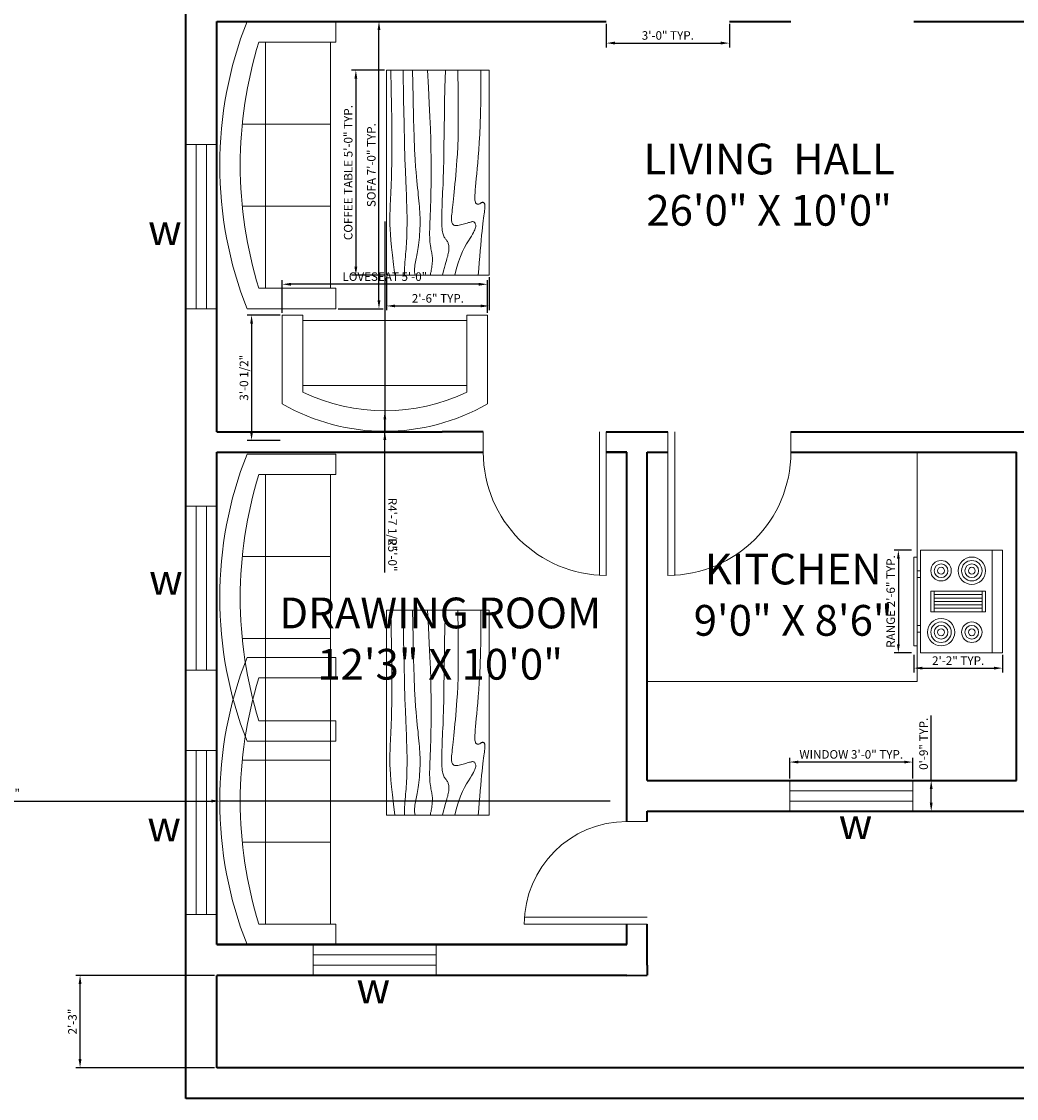
# Model space of a CAD drawing. Units: inches. Extents: x 2009 to 2890, y 2827 to 3504.
# Tile 4 of 6: x 2449 to 2741, y 2899 to 3214. Entities that reach past the tile are written whole.
import ezdxf

# ---------------------------------------------------------------- set-up
doc = ezdxf.new("R2010")
doc.units = ezdxf.units.IN
for name, color, linetype, lineweight in [('A-ANNO-DIMS', 2, 'Continuous', 18), ('A-ANNO-TEXT', 3, 'Continuous', 18), ('A-AREA-IDEN', 7, 'Continuous', 25), ('A-DOOR', 3, 'Continuous', 18), ('A-EQPM', 9, 'Continuous', 18), ('A-FLOR-CASE', 32, 'Continuous', 20), ('A-FURN', 8, 'Continuous', 18), ('A-GLAZ', 4, 'Continuous', 18), ('A-WALL', 7, 'Continuous', 35)]:
    doc.layers.add(name, color=color, linetype=linetype, lineweight=lineweight)
doc.styles.get("Standard").update_dxf_attribs({"font": 'arial.ttf'})
doc.dimstyles.new('ISO-25', dxfattribs={"dimtxt": 2.5, "dimasz": 2.5, "dimexe": 1.25, "dimexo": 0.625, "dimtad": 1, "dimdec": 0, "dimlunit": 3, "dimtxsty": 'Standard', "dimcen": 2.5, "dimadec": 0, "dimazin": 0, "dimtfac": 1, "dimtdec": 0, "dimtmove": 0, "dimatfit": 3, "dimfxl": 1, "dimarcsym": 0})

# ---------------------------------------------------------------- blocks, each defined once
blk = doc.blocks.new('Table - Rectangular Woodgrain 60 x 30 in.')
for p, q in [((0, 0), (0, -30)), ((60, 0), (0, 0)), ((60, -30), (60, 0)), ((0, -30), (60, -30))]:
    blk.add_line(p, q)
for points in [[(0, -2.4), (4.8155, -2.418), (9.0302, -2.4688), (12.709, -2.5477), (15.9167, -2.65), (18.7181, -2.7711), (21.1781, -2.9063), (23.3616, -3.0508), (25.3333, -3.2), (27.1477, -3.3495), (28.8172, -3.4958), (30.3437, -3.636), (31.7291, -3.7667), (32.9756, -3.8849), (34.0849, -3.9875), (35.059, -4.0714), (35.9, -4.1334), (36.6114, -4.1711), (37.2041, -4.1854), (37.6906, -4.1779), (38.0833, -4.15), (38.3948, -4.1034), (38.6375, -4.0396), (38.8239, -3.9602), (38.9666, -3.8667), (39.0764, -3.7608), (39.1573, -3.6448), (39.2116, -3.521), (39.2416, -3.3917), (39.2498, -3.2593), (39.2385, -3.1261), (39.21, -2.9944), (39.1666, -2.8667), (39.111, -2.7447), (39.0468, -2.6281), (38.978, -2.5163), (38.9083, -2.4083), (38.8418, -2.3035), (38.7823, -2.201), (38.7337, -2.1001), (38.7, -2), (38.6844, -1.9003), (38.6875, -1.8021), (38.7094, -1.707), (38.75, -1.6167), (38.8094, -1.5326), (38.8875, -1.4563), (38.9844, -1.3893), (39.1, -1.3333), (39.2351, -1.2896), (39.3937, -1.2583), (39.5804, -1.2396), (39.8, -1.2333), (40.057, -1.2396), (40.3562, -1.2583), (40.7023, -1.2896), (41.1, -1.3333), (41.5547, -1.3895), (42.0755, -1.4573), (42.6721, -1.5361), (43.3542, -1.625), (44.1316, -1.7233), (45.014, -1.8302), (46.0114, -1.9449), (47.1333, -2.0667), (48.3862, -2.1947), (49.7625, -2.3281), (51.2513, -2.4663), (52.8416, -2.6083), (54.5226, -2.7535), (56.2833, -2.9011), (58.1127, -3.0501), (60, -3.2)], [(0, -9.2), (6.5759, -9.0858), (11.9385, -9.0365), (16.2527, -9.0418), (19.6833, -9.0917), (22.3952, -9.1759), (24.5531, -9.2844), (26.322, -9.4069), (27.8666, -9.5333), (29.3241, -9.6553), (30.7203, -9.7719), (32.0532, -9.8837), (33.3208, -9.9917), (34.5213, -10.0965), (35.6526, -10.199), (36.7128, -10.2999), (37.7, -10.4), (38.6129, -10.4996), (39.4531, -10.5969), (40.223, -10.6895), (40.925, -10.775), (41.5613, -10.8512), (42.1344, -10.9156), (42.6465, -10.966), (43.1, -11), (43.4976, -11.0158), (43.8437, -11.0136), (44.143, -10.9942), (44.4, -10.9583), (44.6195, -10.9069), (44.8062, -10.8406), (44.9648, -10.7603), (45.1, -10.6667), (45.2155, -10.5598), (45.3114, -10.4365), (45.3871, -10.2929), (45.4416, -10.125), (45.4743, -9.929), (45.4844, -9.7011), (45.4709, -9.4371), (45.4333, -9.1333), (45.3716, -8.7883), (45.2896, -8.4104), (45.1919, -8.0107), (45.0833, -7.6), (44.9685, -7.1893), (44.8521, -6.7896), (44.7388, -6.4117), (44.6333, -6.0667), (44.54, -5.7628), (44.4614, -5.4979), (44.4001, -5.2675), (44.3583, -5.0667), (44.3384, -4.8909), (44.3427, -4.7354), (44.3736, -4.5956), (44.4333, -4.4667), (44.5236, -4.3453), (44.6427, -4.2333), (44.7884, -4.1339), (44.9583, -4.05), (45.1501, -3.9849), (45.3614, -3.9417), (45.59, -3.9234), (45.8333, -3.9333), (46.0915, -3.9749), (46.3734, -4.0531), (46.6906, -4.1736), (47.0542, -4.3417), (47.4756, -4.5629), (47.9661, -4.8427), (48.5372, -5.1866), (49.2, -5.6), (49.9676, -6.0844), (50.8594, -6.625), (51.8965, -7.2031), (53.1, -7.8), (54.491, -8.3969), (56.0906, -8.975), (57.9199, -9.5156), (60, -10)], [(0, -12.8), (5.1847, -12.9322), (9.6213, -13.0323), (13.3963, -13.1059), (16.5958, -13.1583), (19.3063, -13.1952), (21.614, -13.2219), (23.6054, -13.2439), (25.3666, -13.2667), (26.9728, -13.2947), (28.4531, -13.3281), (29.8256, -13.3663), (31.1083, -13.4083), (32.3191, -13.4535), (33.476, -13.501), (34.597, -13.5501), (35.7, -13.6), (36.7984, -13.6497), (37.8875, -13.6979), (38.9578, -13.743), (40, -13.7833), (41.0047, -13.8174), (41.9625, -13.8438), (42.864, -13.8607), (43.7, -13.8667), (44.4631, -13.8604), (45.1552, -13.8417), (45.7801, -13.8104), (46.3416, -13.7667), (46.8439, -13.7104), (47.2906, -13.6417), (47.6858, -13.5604), (48.0333, -13.4667), (48.3375, -13.3608), (48.6042, -13.2448), (48.8396, -13.121), (49.05, -12.9917), (49.2417, -12.8593), (49.4208, -12.7261), (49.5937, -12.5944), (49.7667, -12.4667), (49.9452, -12.3451), (50.1323, -12.2313), (50.3303, -12.1268), (50.5416, -12.0333), (50.7686, -11.9524), (51.0135, -11.8854), (51.2788, -11.8341), (51.5666, -11.8), (51.8785, -11.7843), (52.2116, -11.7865), (52.562, -11.8059), (52.926, -11.8417), (53.2998, -11.8931), (53.6795, -11.9594), (54.0614, -12.0397), (54.4416, -12.1333), (54.8223, -12.2401), (55.2293, -12.3625), (55.6942, -12.5037), (56.2489, -12.6667), (56.9251, -12.8547), (57.7545, -13.0708), (58.7689, -13.3182), (60, -13.6)], [(0, -18), (5.124, -17.7273), (9.6609, -17.5057), (13.6705, -17.3303), (17.2125, -17.1958), (20.3467, -17.0973), (23.1328, -17.0297), (25.6307, -16.9878), (27.9, -16.9667), (29.9928, -16.9617), (31.9302, -16.9703), (33.7254, -16.9907), (35.3917, -17.0208), (36.9423, -17.0588), (38.3906, -17.1026), (39.7499, -17.1503), (41.0333, -17.2), (42.2519, -17.2496), (43.4073, -17.2969), (44.4986, -17.3395), (45.525, -17.375), (46.4858, -17.4012), (47.3802, -17.4156), (48.2074, -17.416), (48.9667, -17.4), (49.6583, -17.3662), (50.2872, -17.3167), (50.8595, -17.2547), (51.3812, -17.1833), (51.8584, -17.1057), (52.2971, -17.025), (52.7034, -16.9443), (53.0833, -16.8667), (53.443, -16.7951), (53.789, -16.7313), (54.128, -16.6768), (54.4666, -16.6334), (54.8115, -16.6024), (55.1693, -16.5854), (55.5465, -16.5841), (55.95, -16.6), (56.3828, -16.6337), (56.8346, -16.6823), (57.2915, -16.7418), (57.7396, -16.8084), (58.165, -16.878), (58.5539, -16.9469), (58.8924, -17.0111), (59.1666, -17.0667), (59.3679, -17.1107), (59.5078, -17.1438), (59.6032, -17.1675), (59.6708, -17.1833), (59.7275, -17.193), (59.7901, -17.1979), (59.8753, -17.1998), (60, -17.2)], [(0, -22.4), (8.0098, -22.2501), (14.4094, -22.1011), (19.4168, -21.9535), (23.25, -21.8083), (26.1269, -21.6663), (28.2656, -21.5281), (29.884, -21.3947), (31.2, -21.2667), (32.3967, -21.1448), (33.5172, -21.0292), (34.5697, -20.9198), (35.5625, -20.8167), (36.5037, -20.7198), (37.4015, -20.6292), (38.2642, -20.5448), (39.1, -20.4667), (39.9164, -20.3951), (40.7187, -20.3313), (41.5117, -20.2768), (42.3, -20.2333), (43.0883, -20.2024), (43.8812, -20.1854), (44.6836, -20.1841), (45.5, -20.2), (46.3328, -20.234), (47.1747, -20.2844), (48.0163, -20.3488), (48.8479, -20.425), (49.66, -20.5106), (50.4429, -20.6031), (51.1872, -20.7004), (51.8833, -20.8), (52.5246, -20.8999), (53.1166, -20.9995), (53.6681, -21.0983), (54.1875, -21.1958), (54.6834, -21.2919), (55.1646, -21.3859), (55.6394, -21.4777), (56.1167, -21.5667), (56.6028, -21.6515), (57.0961, -21.7266), (57.5929, -21.7852), (58.0896, -21.8208), (58.5823, -21.8268), (59.0674, -21.7964), (59.5412, -21.723), (60, -21.6)], [(0, -25.2), (8.6355, -25.0504), (15.7026, -24.9031), (21.4049, -24.7606), (25.9458, -24.625), (29.529, -24.4988), (32.3578, -24.3844), (34.6359, -24.284), (36.5667, -24.2), (38.3213, -24.1341), (39.9417, -24.0854), (41.437, -24.0523), (42.8167, -24.0333), (44.0901, -24.0268), (45.2667, -24.0313), (46.3557, -24.0451), (47.3667, -24.0667), (48.309, -24.0947), (49.1928, -24.1287), (50.0284, -24.168), (50.826, -24.2125), (51.5959, -24.2617), (52.3483, -24.3151), (53.0935, -24.3725), (53.8417, -24.4334), (54.6009, -24.497), (55.3699, -24.561), (56.1454, -24.6226), (56.9239, -24.6792), (57.7021, -24.7279), (58.4764, -24.7662), (59.2435, -24.7911), (60, -24.8)], [(0, -28.8), (5.6867, -28.6681), (10.45, -28.5698), (14.407, -28.5012), (17.675, -28.4584), (20.3711, -28.4374), (22.6125, -28.4344), (24.5164, -28.4455), (26.2, -28.4667), (27.762, -28.4947), (29.2276, -28.5281), (30.6033, -28.5663), (31.8958, -28.6084), (33.1118, -28.6535), (34.2578, -28.7011), (35.3405, -28.7501), (36.3666, -28.8), (37.3443, -28.8497), (38.288, -28.8974), (39.2137, -28.9412), (40.1375, -28.9792), (41.0753, -29.0093), (42.0432, -29.0297), (43.0572, -29.0384), (44.1333, -29.0333), (45.2936, -29.0114), (46.5843, -28.9641), (48.0579, -28.8816), (49.7666, -28.7542), (51.7629, -28.5721), (54.0989, -28.3255), (56.8272, -28.0048), (60, -27.6)]]:
    blk.add_lwpolyline(points)
blk = doc.blocks.new('Sofa - Roundback 7 ft.')
for p, q in [((-12.00002, -32.4421), (-12.00003, -6.5971)), ((11.99997, -32.4421), (11.99998, -6.5971)), ((-36.000027, -34), (-36.000027, -11.4696)), ((35.99998, -34), (35.99998, -11.4696)), ((-35.999844, -13.3819), (35.9998, -13.3819)), ((-36.000027, -32.4421), (35.99998, -32.4421))]:
    blk.add_line(p, q)
for points in [[(-36.000027, -34), (-42.000027, -34), (-42.000027, -8)], [(41.99998, -8), (41.99998, -34), (35.99998, -34)]]:
    blk.add_lwpolyline(points)
for centre, radius, start, end in [((0, -114.25), 114.25, 68.43141, 111.5686), ((-0.00001, -127.1968), 121.1968, 72.72033, 107.2797)]:
    blk.add_arc(centre, radius, start, end)
blk = doc.blocks.new('Sofa - Roundback Loveseat 5 ft.')
for p, q in [((0, -32.44198), (0, -5.99998)), ((-24, -33.99998), (-24, -11.46958)), ((24.00004, -33.99998), (24.00004, -11.46958)), ((-23.9998, -13.38178), (23.99986, -13.38178)), ((-24, -32.44198), (24.00004, -32.44198))]:
    blk.add_line(p, q)
for points in [[(-24, -33.99998), (-30, -33.99998), (-30, -7.99998)], [(30.00004, -7.99998), (30.00004, -33.99998), (24.00004, -33.99998)]]:
    blk.add_lwpolyline(points)
for centre, radius, start, end in [((0, -60.24998), 60.24998, 60.13715, 119.8628), ((0, -61.38438), 55.38444, 64.32083, 115.6792)]:
    blk.add_arc(centre, radius, start, end)
blk = doc.blocks.new('Range-Oven - 30 in top')
for p, q in [((0, -3), (30, -3)), ((12, -6), (18, -6)), ((13, -20), (13, -6)), ((14, -6), (14, -20)), ((15, -20), (15, -6)), ((16, -6), (16, -20)), ((17, -20), (17, -6)), ((18, -20), (12, -20)), ((6, -24), (6, -25)), ((8, -25), (8, -24)), ((22, -25), (22, -24)), ((24, -24), (24, -25))]:
    blk.add_line(p, q)
for points in [[(0, -24), (0, 0), (30, 0), (30, -24)], [(12, -21), (12, -5), (18, -5), (18, -21)], [(2, -26), (2, -25), (28, -25), (28, -26)]]:
    blk.add_lwpolyline(points, close=True)
for centre, radius in [((6, -9), 4), ((6, -9), 3), ((24, -9), 3), ((6, -9), 2), ((6, -9), 1), ((24, -9), 2), ((24, -9), 1), ((6, -18), 3), ((24, -18), 4), ((24, -18), 3), ((6, -18), 2), ((6, -18), 1), ((24, -18), 2), ((24, -18), 1)]:
    blk.add_circle(centre, radius)
blk = doc.blocks.new('WIN-48IN')
for p, q in [((0, 48), (0, 0)), ((9, 48), (0, 48)), ((3, 48), (3, 0)), ((6, 0), (6, 48)), ((9, 0), (9, 48)), ((0, 0), (9, 0))]:
    blk.add_line(p, q)
blk = doc.blocks.new('WIN-36IN')
for p, q in [((0, 36), (0, 0)), ((9, 36), (0, 36)), ((3, 36), (3, 0)), ((6, 0), (6, 36)), ((9, 0), (9, 36)), ((0, 0), (9, 0))]:
    blk.add_line(p, q)
blk = doc.blocks.new('DOOR-36IN')
for p, q in [((34, 6), (34, 42)), ((36, 6), (36, 42)), ((0, 0), (0, 6)), ((34, 6), (34, 0)), ((36, 6), (36, 0))]:
    blk.add_line(p, q)
blk.add_arc((36, 6), 36, 90, 180)
blk = doc.blocks.new('DOOR-30IN')
for p, q in [((0, 2), (30, 2)), ((0, 0), (30, 0))]:
    blk.add_line(p, q)
blk.add_arc((0, 0), 30, 0, 90)
blk = doc.blocks.new('*D33')
at = {"layer": 'A-ANNO-DIMS', "color": 0, "lineweight": -2, "transparency": 16777216}
for p, q in [((2674.28, 2992.57), (2674.28, 2998.59)), ((2707.78, 2997.34), (2676.78, 2997.34)), ((2710.28, 2992.57), (2710.28, 2998.59))]:
    blk.add_line(p, q, dxfattribs=at)
at = {"layer": 'A-ANNO-DIMS', "color": 0, "transparency": 16777216}
for points in [[(2676.78, 2997.76), (2676.78, 2996.93), (2674.28, 2997.34)], [(2707.78, 2997.76), (2707.78, 2996.93), (2710.28, 2997.34)]]:
    blk.add_solid(points, dxfattribs=at)
at = {"layer": 'Defpoints', "color": 0, "transparency": 16777216}
for p in [(2674.28, 2997.34), (2674.28, 2991.94), (2710.28, 2991.94)]:
    blk.add_point(p, dxfattribs=at)
at = {"layer": 'A-ANNO-DIMS', "color": 0, "transparency": 16777216, "insert": (2692.28, 2999.26), "char_height": 2.5, "attachment_point": 5}
blk.add_mtext('WINDOW 3\'-0" TYP.', dxfattribs=at)
blk = doc.blocks.new('*D34')
at = {"layer": 'A-ANNO-DIMS', "color": 0, "lineweight": -2, "transparency": 16777216}
for p, q in [((2715.68, 2991.94), (2715.68, 3010.93)), ((2710.9, 2991.94), (2716.93, 2991.94)), ((2715.68, 2985.44), (2715.68, 2989.44)), ((2710.9, 2982.94), (2716.93, 2982.94))]:
    blk.add_line(p, q, dxfattribs=at)
at = {"layer": 'A-ANNO-DIMS', "color": 0, "transparency": 16777216}
for points in [[(2715.26, 2989.44), (2716.09, 2989.44), (2715.68, 2991.94)], [(2715.26, 2985.44), (2716.09, 2985.44), (2715.68, 2982.94)]]:
    blk.add_solid(points, dxfattribs=at)
at = {"layer": 'Defpoints', "color": 0, "transparency": 16777216}
for p in [(2710.28, 2991.94), (2715.68, 2991.94), (2710.28, 2982.94)]:
    blk.add_point(p, dxfattribs=at)
at = {"layer": 'A-ANNO-DIMS', "color": 0, "transparency": 16777216, "insert": (2713.77, 3002.69), "char_height": 2.5, "attachment_point": 5, "rotation": 90}
blk.add_mtext('0\'-9" TYP.', dxfattribs=at)
blk = doc.blocks.new('*D38')
at = {"layer": 'A-ANNO-DIMS', "color": 0, "lineweight": -2, "transparency": 16777216}
for p, q in [((2620.61, 3213.32), (2620.61, 3206.39)), ((2656.61, 3213.32), (2656.61, 3206.39)), ((2623.11, 3207.64), (2654.11, 3207.64))]:
    blk.add_line(p, q, dxfattribs=at)
at = {"layer": 'A-ANNO-DIMS', "color": 0, "transparency": 16777216}
for points in [[(2623.11, 3208.06), (2623.11, 3207.23), (2620.61, 3207.64)], [(2654.11, 3208.06), (2654.11, 3207.23), (2656.61, 3207.64)]]:
    blk.add_solid(points, dxfattribs=at)
at = {"layer": 'Defpoints', "color": 0, "transparency": 16777216}
for p in [(2620.61, 3213.94), (2656.61, 3213.94), (2656.61, 3207.64)]:
    blk.add_point(p, dxfattribs=at)
at = {"layer": 'A-ANNO-DIMS', "color": 0, "transparency": 16777216, "insert": (2638.61, 3209.55), "char_height": 2.5, "attachment_point": 5}
blk.add_mtext('3\'-0" TYP.', dxfattribs=at)
blk = doc.blocks.new('*D51')
at = {"layer": 'A-ANNO-DIMS', "color": 0, "lineweight": -2, "transparency": 16777216}
for p, q in [((2542.11, 3213.94), (2555.33, 3213.94)), ((2554.08, 3132.44), (2554.08, 3211.44)), ((2542.11, 3129.94), (2555.33, 3129.94))]:
    blk.add_line(p, q, dxfattribs=at)
at = {"layer": 'A-ANNO-DIMS', "color": 0, "transparency": 16777216}
for points in [[(2553.67, 3211.44), (2554.5, 3211.44), (2554.08, 3213.94)], [(2553.67, 3132.44), (2554.5, 3132.44), (2554.08, 3129.94)]]:
    blk.add_solid(points, dxfattribs=at)
at = {"layer": 'Defpoints', "color": 0, "transparency": 16777216}
for p in [(2541.48, 3213.94), (2554.08, 3213.94), (2541.48, 3129.94)]:
    blk.add_point(p, dxfattribs=at)
at = {"layer": 'A-ANNO-DIMS', "color": 0, "transparency": 16777216, "insert": (2552.16, 3171.94), "char_height": 2.5, "attachment_point": 5, "rotation": 90}
blk.add_mtext('SOFA 7\'-0" TYP.', dxfattribs=at)
blk = doc.blocks.new('*D53')
at = {"layer": 'A-ANNO-DIMS', "color": 0, "lineweight": -2, "transparency": 16777216}
for p, q in [((2525.8, 3128.72), (2525.8, 3138.34)), ((2585.8, 3128.72), (2585.8, 3138.34)), ((2583.3, 3137.09), (2528.3, 3137.09))]:
    blk.add_line(p, q, dxfattribs=at)
at = {"layer": 'A-ANNO-DIMS', "color": 0, "transparency": 16777216}
for points in [[(2528.3, 3137.51), (2528.3, 3136.68), (2525.8, 3137.09)], [(2583.3, 3137.51), (2583.3, 3136.68), (2585.8, 3137.09)]]:
    blk.add_solid(points, dxfattribs=at)
at = {"layer": 'Defpoints', "color": 0, "transparency": 16777216}
for p in [(2525.8, 3137.09), (2525.8, 3128.09), (2585.8, 3128.09)]:
    blk.add_point(p, dxfattribs=at)
at = {"layer": 'A-ANNO-DIMS', "color": 0, "transparency": 16777216, "insert": (2555.8, 3139.01), "char_height": 2.5, "attachment_point": 5}
blk.add_mtext('LOVESEAT 5\'-0"', dxfattribs=at)
blk = doc.blocks.new('*D54')
at = {"layer": 'A-ANNO-DIMS', "color": 0, "lineweight": -2, "transparency": 16777216}
for p, q in [((2525.18, 3128.09), (2515.55, 3128.09)), ((2516.8, 3125.59), (2516.8, 3093.93)), ((2525.18, 3091.43), (2515.55, 3091.43))]:
    blk.add_line(p, q, dxfattribs=at)
at = {"layer": 'A-ANNO-DIMS', "color": 0, "transparency": 16777216}
for points in [[(2516.39, 3125.59), (2517.22, 3125.59), (2516.8, 3128.09)], [(2516.39, 3093.93), (2517.22, 3093.93), (2516.8, 3091.43)]]:
    blk.add_solid(points, dxfattribs=at)
at = {"layer": 'Defpoints', "color": 0, "transparency": 16777216}
for p in [(2525.8, 3128.09), (2516.8, 3091.43), (2525.8, 3091.43)]:
    blk.add_point(p, dxfattribs=at)
at = {"layer": 'A-ANNO-DIMS', "color": 0, "transparency": 16777216, "insert": (2514.89, 3109.76), "char_height": 2.5, "attachment_point": 5, "rotation": 90}
blk.add_mtext('3\'-0 1/2"', dxfattribs=at)
blk = doc.blocks.new('*D55')
at = {"layer": 'A-ANNO-DIMS', "color": 0, "lineweight": -2, "transparency": 16777216}
for p, q in [((2555.7, 3199.75), (2546.07, 3199.75)), ((2547.32, 3197.25), (2547.32, 3142.25)), ((2555.7, 3139.75), (2546.07, 3139.75))]:
    blk.add_line(p, q, dxfattribs=at)
at = {"layer": 'A-ANNO-DIMS', "color": 0, "transparency": 16777216}
for points in [[(2546.9, 3197.25), (2547.74, 3197.25), (2547.32, 3199.75)], [(2546.9, 3142.25), (2547.74, 3142.25), (2547.32, 3139.75)]]:
    blk.add_solid(points, dxfattribs=at)
at = {"layer": 'Defpoints', "color": 0, "transparency": 16777216}
for p in [(2556.32, 3199.75), (2547.32, 3139.75), (2556.32, 3139.75)]:
    blk.add_point(p, dxfattribs=at)
at = {"layer": 'A-ANNO-DIMS', "color": 0, "transparency": 16777216, "insert": (2545.4, 3169.75), "char_height": 2.5, "attachment_point": 5, "rotation": 90}
blk.add_mtext('COFFEE TABLE 5\'-0" TYP.', dxfattribs=at)
blk = doc.blocks.new('*D56')
at = {"layer": 'A-ANNO-DIMS', "color": 0, "lineweight": -2, "transparency": 16777216}
for p, q in [((2556.32, 3139.13), (2556.32, 3129.5)), ((2586.32, 3139.13), (2586.32, 3129.5)), ((2558.82, 3130.75), (2583.82, 3130.75))]:
    blk.add_line(p, q, dxfattribs=at)
at = {"layer": 'A-ANNO-DIMS', "color": 0, "transparency": 16777216}
for points in [[(2558.82, 3131.17), (2558.82, 3130.34), (2556.32, 3130.75)], [(2583.82, 3131.17), (2583.82, 3130.34), (2586.32, 3130.75)]]:
    blk.add_solid(points, dxfattribs=at)
at = {"layer": 'Defpoints', "color": 0, "transparency": 16777216}
for p in [(2556.32, 3139.75), (2586.32, 3139.75), (2586.32, 3130.75)]:
    blk.add_point(p, dxfattribs=at)
at = {"layer": 'A-ANNO-DIMS', "color": 0, "transparency": 16777216, "insert": (2571.32, 3132.65), "char_height": 2.5, "attachment_point": 5}
blk.add_mtext('2\'-6" TYP.', dxfattribs=at)
blk = doc.blocks.new('*D57')
at = {"layer": 'A-ANNO-DIMS', "color": 0, "lineweight": -2, "transparency": 16777216}
for p, q in [((2709.94, 3059.31), (2704.81, 3059.31)), ((2706.06, 3056.81), (2706.06, 3031.81)), ((2709.94, 3029.31), (2704.81, 3029.31))]:
    blk.add_line(p, q, dxfattribs=at)
at = {"layer": 'A-ANNO-DIMS', "color": 0, "transparency": 16777216}
for points in [[(2705.65, 3056.81), (2706.48, 3056.81), (2706.06, 3059.31)], [(2705.65, 3031.81), (2706.48, 3031.81), (2706.06, 3029.31)]]:
    blk.add_solid(points, dxfattribs=at)
at = {"layer": 'Defpoints', "color": 0, "transparency": 16777216}
for p in [(2710.56, 3059.31), (2706.06, 3029.31), (2710.56, 3029.31)]:
    blk.add_point(p, dxfattribs=at)
at = {"layer": 'A-ANNO-DIMS', "color": 0, "transparency": 16777216, "insert": (2704.15, 3044.31), "char_height": 2.5, "attachment_point": 5, "rotation": 90}
blk.add_mtext('RANGE 2\'-6" TYP.', dxfattribs=at)
blk = doc.blocks.new('*D58')
at = {"layer": 'A-ANNO-DIMS', "color": 0, "lineweight": -2, "transparency": 16777216}
for p, q in [((2710.56, 3028.69), (2710.56, 3023.56)), ((2736.56, 3028.69), (2736.56, 3023.56)), ((2713.06, 3024.81), (2734.06, 3024.81))]:
    blk.add_line(p, q, dxfattribs=at)
at = {"layer": 'A-ANNO-DIMS', "color": 0, "transparency": 16777216}
for points in [[(2713.06, 3025.23), (2713.06, 3024.4), (2710.56, 3024.81)], [(2734.06, 3025.23), (2734.06, 3024.4), (2736.56, 3024.81)]]:
    blk.add_solid(points, dxfattribs=at)
at = {"layer": 'Defpoints', "color": 0, "transparency": 16777216}
for p in [(2710.56, 3029.31), (2736.56, 3029.31), (2736.56, 3024.81)]:
    blk.add_point(p, dxfattribs=at)
at = {"layer": 'A-ANNO-DIMS', "color": 0, "transparency": 16777216, "insert": (2723.56, 3026.69), "char_height": 2.5, "attachment_point": 5}
blk.add_mtext('2\'-2" TYP.', dxfattribs=at)
blk = doc.blocks.new('*D74')
at = {"layer": 'A-ANNO-DIMS', "color": 0, "lineweight": -2, "transparency": 16777216}
for p, q in [((2505.99, 2934.94), (2465.36, 2934.94)), ((2466.61, 2910.44), (2466.61, 2932.44)), ((2505.99, 2907.94), (2465.36, 2907.94))]:
    blk.add_line(p, q, dxfattribs=at)
at = {"layer": 'A-ANNO-DIMS', "color": 0, "transparency": 16777216}
for points in [[(2466.19, 2932.44), (2467.03, 2932.44), (2466.61, 2934.94)], [(2466.19, 2910.44), (2467.03, 2910.44), (2466.61, 2907.94)]]:
    blk.add_solid(points, dxfattribs=at)
at = {"layer": 'Defpoints', "color": 0, "transparency": 16777216}
for p in [(2466.61, 2934.94), (2506.61, 2934.94), (2506.61, 2907.94)]:
    blk.add_point(p, dxfattribs=at)
at = {"layer": 'A-ANNO-DIMS', "color": 0, "transparency": 16777216, "insert": (2464.71, 2921.44), "char_height": 2.5, "attachment_point": 5, "rotation": 90}
blk.add_mtext('2\'-3"', dxfattribs=at)
blk = doc.blocks.new('*D87')
at = {"layer": 'A-ANNO-DIMS', "color": 0, "lineweight": -2, "transparency": 16777216}
for p, q in [((2428.19, 2985.94), (2504.98, 2985.94)), ((2621.73, 2985.94), (2507.48, 2985.94))]:
    blk.add_line(p, q, dxfattribs=at)
at = {"layer": 'A-ANNO-DIMS', "color": 0, "transparency": 16777216}
blk.add_solid([(2504.98, 2986.36), (2504.98, 2985.53), (2507.48, 2985.94)], dxfattribs=at)
at = {"layer": 'Defpoints', "color": 0, "transparency": 16777216}
for p in [(2507.48, 2985.94), (2621.73, 2985.94)]:
    blk.add_point(p, dxfattribs=at)
at = {"layer": 'A-ANNO-DIMS', "color": 0, "transparency": 16777216, "insert": (2438.93, 2987.86), "char_height": 2.5, "attachment_point": 5, "rotation": 0.0001}
blk.add_mtext('5X R9\'-6 1/2"', dxfattribs=at)
blk = doc.blocks.new('*D88')
at = {"layer": 'A-ANNO-DIMS', "color": 0, "lineweight": -2, "transparency": 16777216}
for p, q in [((2555.8, 3154.34), (2555.8, 3094.09)), ((2555.8, 3052.8), (2555.8, 3091.59))]:
    blk.add_line(p, q, dxfattribs=at)
at = {"layer": 'A-ANNO-DIMS', "color": 0, "transparency": 16777216}
blk.add_solid([(2556.22, 3091.59), (2555.39, 3091.59), (2555.8, 3094.09)], dxfattribs=at)
at = {"layer": 'Defpoints', "color": 0, "transparency": 16777216}
for p in [(2555.8, 3154.34), (2555.8, 3094.09)]:
    blk.add_point(p, dxfattribs=at)
at = {"layer": 'A-ANNO-DIMS', "color": 0, "transparency": 16777216, "insert": (2557.71, 3057.94), "char_height": 2.5, "attachment_point": 5, "rotation": 270.0001}
blk.add_mtext('R5\'-0"', dxfattribs=at)
blk = doc.blocks.new('*D89')
at = {"layer": 'A-ANNO-DIMS', "color": 0, "lineweight": -2, "transparency": 16777216}
for p, q in [((2555.8, 3155.48), (2555.8, 3100.09)), ((2555.8, 3058.8), (2555.8, 3097.59))]:
    blk.add_line(p, q, dxfattribs=at)
at = {"layer": 'A-ANNO-DIMS', "color": 0, "transparency": 16777216}
blk.add_solid([(2556.22, 3097.59), (2555.39, 3097.59), (2555.8, 3100.09)], dxfattribs=at)
at = {"layer": 'Defpoints', "color": 0, "transparency": 16777216}
for p in [(2555.8, 3155.48), (2555.8, 3100.09)]:
    blk.add_point(p, dxfattribs=at)
at = {"layer": 'A-ANNO-DIMS', "color": 0, "transparency": 16777216, "insert": (2557.72, 3066.86), "char_height": 2.5, "attachment_point": 5, "rotation": 270.0001}
blk.add_mtext('R4\'-7 1/2"', dxfattribs=at)

msp = doc.modelspace()

# ---------------------------------------------------------------- linework, layer by layer
at = {"layer": 'A-DOOR'}
for p, q in [((2620.61, 3087.94), (2620.61, 3093.94)), ((2620.61, 3087.94), (2620.61, 3093.94)), ((2632.61, 2979.94), (2626.61, 2979.94)), ((2626.61, 2951.94), (2632.61, 2951.94)), ((2626.61, 2949.94), (2632.61, 2949.94))]:
    msp.add_line(p, q, dxfattribs=at)
msp.add_circle((2584.61, 3087.94), 4.547e-13, dxfattribs=at)
at = {"layer": 'A-FLOR-CASE'}
for p, q in [((2711.61, 3020.94), (2711.61, 3087.94)), ((2632.61, 3020.94), (2711.61, 3020.94))]:
    msp.add_line(p, q, dxfattribs=at)
at = {"layer": 'A-GLAZ'}
for p, q in [((2674.28, 2985.94), (2710.28, 2985.94)), ((2534.86, 2937.94), (2570.86, 2937.94))]:
    msp.add_line(p, q, dxfattribs=at)
at = {"layer": 'A-WALL'}
for p, q in [((2497.61, 2898.94), (2497.61, 3438.94)), ((2506.61, 3213.94), (2620.61, 3213.94)), ((2506.61, 3093.94), (2506.61, 3213.94)), ((2656.61, 3213.94), (2674.61, 3213.94)), ((2710.61, 3213.94), (2848.61, 3213.94)), ((2506.61, 3093.94), (2572.61, 3093.94)), ((2584.61, 3093.94), (2572.61, 3093.94)), ((2620.61, 3093.94), (2638.61, 3093.94)), ((2674.61, 3093.94), (2752.61, 3093.94)), ((2506.61, 3087.94), (2572.61, 3087.94)), ((2506.61, 2943.94), (2506.61, 3087.94)), ((2572.61, 3087.94), (2584.61, 3087.94)), ((2626.61, 3087.94), (2620.61, 3087.94)), ((2620.61, 3087.94), (2626.61, 3087.94)), ((2626.61, 2979.94), (2626.61, 3087.94)), ((2632.61, 3087.94), (2638.61, 3087.94)), ((2632.61, 2991.94), (2632.61, 3087.94)), ((2632.61, 3087.94), (2638.61, 3087.94)), ((2674.61, 3087.94), (2740.61, 3087.94)), ((2740.61, 2991.94), (2740.61, 3087.94)), ((2632.61, 2991.94), (2740.61, 2991.94)), ((2632.61, 2979.94), (2632.61, 2982.94)), ((2632.61, 2982.94), (2740.61, 2982.94)), ((2740.61, 2982.94), (2746.61, 2982.94)), ((2626.61, 2943.94), (2626.61, 2949.94)), ((2626.61, 2943.94), (2626.61, 2949.94)), ((2632.61, 2937.94), (2632.61, 2949.94)), ((2506.61, 2943.94), (2626.61, 2943.94)), ((2626.61, 2943.94), (2506.61, 2943.94)), ((2632.61, 2937.94), (2632.61, 2934.98)), ((2506.61, 2907.94), (2506.61, 2934.94)), ((2626.61, 2934.94), (2506.61, 2934.94)), ((2626.61, 2934.94), (2632.61, 2934.98)), ((2848.61, 2907.94), (2506.61, 2907.94)), ((2857.61, 2898.94), (2497.61, 2898.94))]:
    msp.add_line(p, q, dxfattribs=at)

# ---------------------------------------------------------------- block references
at = {"layer": 'A-DOOR', "extrusion": (0, 0, -1), "zscale": -1, "rotation": 180}
msp.add_blockref('DOOR-36IN', (-2584.61, 3093.94), dxfattribs=at)
at = {"layer": 'A-DOOR', "rotation": 180}
msp.add_blockref('DOOR-36IN', (2674.61, 3093.94), dxfattribs=at)
at = {"layer": 'A-DOOR', "extrusion": (0, 0, -1), "zscale": -1}
msp.add_blockref('DOOR-30IN', (-2626.61, 2949.94), dxfattribs=at)
at = {"layer": 'A-EQPM', "rotation": 270}
msp.add_blockref('Range-Oven - 30 in top', (2736.56, 3059.31), dxfattribs=at)
at = {"layer": 'A-FURN'}
for name, p, rotation in [('Sofa - Roundback 7 ft.', (2507.48, 3171.94), 90), ('Table - Rectangular Woodgrain 60 x 30 in.', (2586.32, 3199.75), 270.0000000000006), ('Sofa - Roundback Loveseat 5 ft.', (2555.8, 3094.09), 180), ('Sofa - Roundback 7 ft.', (2507.48, 3045.44), 90), ('Table - Rectangular Woodgrain 60 x 30 in.', (2586.32, 3041.81), 270.0000000000006), ('Sofa - Roundback 7 ft.', (2507.48, 2985.94), 90)]:
    msp.add_blockref(name, p, dxfattribs=dict(at, rotation=rotation))
at = {"layer": 'A-GLAZ'}
for p in [(2497.61, 3129.94), (2497.61, 3024.23), (2497.61, 2952.73)]:
    msp.add_blockref('WIN-48IN', p, dxfattribs=at)
at = {"layer": 'A-GLAZ', "rotation": 89.9999999999993}
for p in [(2710.28, 2982.94), (2570.86, 2934.94)]:
    msp.add_blockref('WIN-36IN', p, dxfattribs=at)

# ---------------------------------------------------------------- texts
at = {"layer": 'A-ANNO-TEXT', "char_height": 9, "attachment_point": 1}
for insert in [(2464.62, 3157.57), (2464.91, 3055.26), (2464.39, 2983.13), (2666.7, 2983.83), (2525.6, 2935.79)]:
    msp.add_mtext_dynamic_manual_height_columns('\\pxqc;w', width=53.6341, gutter_width=12.5, heights=[0], dxfattribs=dict(at, insert=insert))
at = {"layer": 'A-AREA-IDEN', "char_height": 9, "attachment_point": 1}
for s, width, insert in [('\\pxqc;LIVING  HALL\\P26\'0" X 10\'0"', 102.762, (2616.88, 3178.23)), ('\\pxqc;KITCHEN\\P9\'0" X 8\'6"', 97.3998, (2626.61, 3058.29)), ('\\pxqc;DRAWING ROOM\\P12\'3" X 10\'0"', 123.1458, (2510.42, 3045.45))]:
    msp.add_mtext_dynamic_manual_height_columns(s, width=width, gutter_width=12.5, heights=[0], dxfattribs=dict(at, insert=insert))

# ---------------------------------------------------------------- dimensions: what is measured, and where the dimension line sits
at = {"layer": 'A-ANNO-DIMS'}
for base, p1, p2, angle, text, picture, middle in [((2554.08, 3213.94), (2541.48, 3129.94), (2541.48, 3213.94), 90, 'SOFA <> TYP.', '*D51', (2552.16, 3171.94)), ((2547.32, 3139.75), (2556.32, 3199.75), (2556.32, 3139.75), 270, 'COFFEE TABLE <> TYP.', '*D55', (2545.4, 3169.75)), ((2525.8, 3137.09), (2585.8, 3128.09), (2525.8, 3128.09), 180, 'LOVESEAT <>', '*D53', (2555.8, 3139.01)), ((2586.32, 3130.75), (2556.32, 3139.75), (2586.32, 3139.75), 0, '<> TYP.', '*D56', (2571.32, 3132.65)), ((2706.06, 3029.31), (2710.56, 3059.31), (2710.56, 3029.31), 270, 'RANGE <> TYP.', '*D57', (2704.15, 3044.31)), ((2715.68, 2991.94), (2710.28, 2982.94), (2710.28, 2991.94), 90, '<> TYP.', '*D34', (2713.77, 3002.69)), ((2674.28, 2997.34), (2710.28, 2991.94), (2674.28, 2991.94), 180, 'WINDOW <> TYP.', '*D33', (2692.28, 2999.26))]:
    dim = msp.add_linear_dim(base=base, p1=p1, p2=p2, angle=angle, text=text, dimstyle='ISO-25', override={"dimdec": 1, "dimlfac": 1, "dimrnd": 0, "dimzin": 1, "dimdsep": 46, "dimlunit": 4, "dimfrac": 2}, dxfattribs=at)
    dim.commit()
    dim.dimension.update_dxf_attribs({"geometry": picture, "text_midpoint": middle})
for base, p1, p2, picture, middle in [((2656.61, 3207.64), (2620.61, 3213.94), (2656.61, 3213.94), '*D38', (2638.61, 3209.55)), ((2736.56, 3024.81), (2710.56, 3029.31), (2736.56, 3029.31), '*D58', (2723.56, 3026.69))]:
    dim = msp.add_linear_dim(base=base, p1=p1, p2=p2, text='<> TYP.', dimstyle='ISO-25', override={"dimdec": 1, "dimlfac": 1, "dimrnd": 0, "dimzin": 1, "dimdsep": 46, "dimlunit": 4, "dimfrac": 2}, dxfattribs=at)
    dim.commit()
    dim.dimension.update_dxf_attribs({"geometry": picture, "text_midpoint": middle})
for center, mpoint, picture, middle in [((2555.8, 3155.48), (2555.8, 3100.09), '*D89', (2555.8, 3066.86)), ((2555.80391, 3154.34203), (2555.804, 3094.09205), '*D88', (2555.80406, 3057.94206))]:
    dim = msp.add_radius_dim(center=center, mpoint=mpoint, dimstyle='ISO-25', override={"dimdec": 1, "dimlfac": 1, "dimrnd": 0, "dimzin": 1, "dimdsep": 46, "dimlunit": 4, "dimfrac": 2}, dxfattribs=at)
    dim.commit()
    dim.dimension.update_dxf_attribs({"geometry": picture, "text_midpoint": middle, "dimtype": 164})
for base, p1, p2, angle, picture, middle in [((2516.8, 3091.43), (2525.8, 3128.09), (2525.8, 3091.43), 270, '*D54', (2514.89, 3109.76)), ((2466.61, 2934.94), (2506.61, 2907.94), (2506.61, 2934.94), 90, '*D74', (2464.71, 2921.44))]:
    dim = msp.add_linear_dim(base=base, p1=p1, p2=p2, angle=angle, dimstyle='ISO-25', override={"dimdec": 1, "dimlfac": 1, "dimrnd": 0, "dimzin": 1, "dimdsep": 46, "dimlunit": 4, "dimfrac": 2}, dxfattribs=at)
    dim.commit()
    dim.dimension.update_dxf_attribs({"geometry": picture, "text_midpoint": middle})
dim = msp.add_radius_dim(center=(2621.732653, 2985.944293), mpoint=(2507.482653, 2985.944), text='5X <>', dimstyle='ISO-25', override={"dimdec": 1, "dimlfac": 1, "dimrnd": 0, "dimzin": 1, "dimdsep": 46, "dimlunit": 4, "dimfrac": 2}, dxfattribs=at)
dim.commit()
dim.dimension.update_dxf_attribs({"geometry": '*D87', "text_midpoint": (2438.932653, 2985.9438242), "dimtype": 164})

doc.saveas('drawing.dxf')
